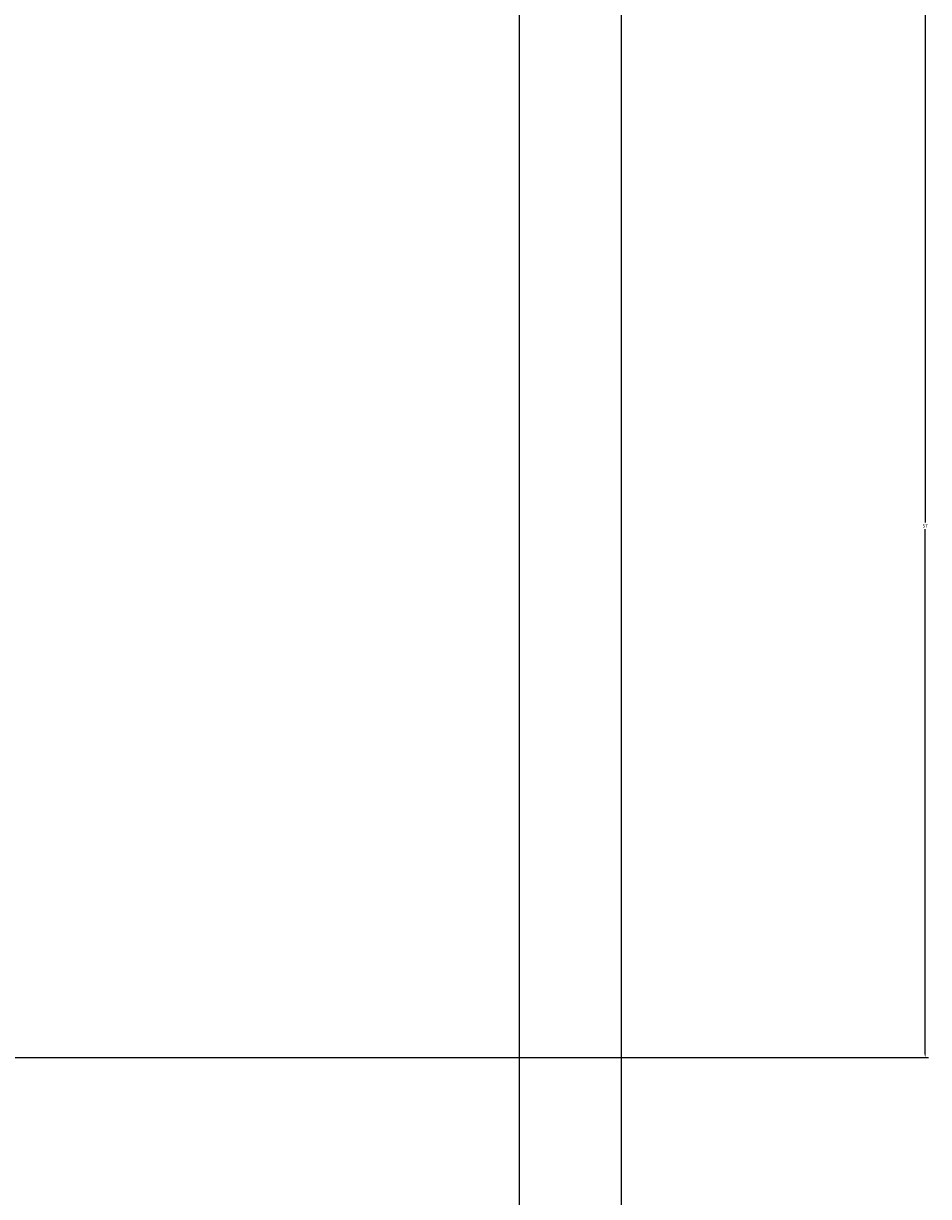
# Model space of a CAD drawing. Units: inches. Extents: x 84 to 1044, y -280 to 906.
# Tile 46 of 105: x 995 to 1044, y -129 to -66. Entities that reach past the tile are written whole.
import ezdxf

# ---------------------------------------------------------------- set-up
doc = ezdxf.new("R2010")
doc.units = ezdxf.units.IN
doc.layers.add('A-ANNO-DIMS', color=2, linetype='Continuous', lineweight=18)
doc.layers.add('A-ANNO-TTLB', color=7, linetype='Continuous', lineweight=25)
doc.styles.get("Standard").update_dxf_attribs({"font": 'arial.ttf'})
doc.dimstyles.get("Standard").update_dxf_attribs({"dimtxt": 0.18, "dimasz": 0.18, "dimexe": 0.18, "dimexo": 0.0625, "dimgap": 0.09, "dimtad": 0, "dimtih": 1, "dimtoh": 1, "dimdec": 4, "dimzin": 0, "dimdsep": 46, "dimtxsty": 'Standard', "dimcen": 0.09, "dimadec": 0, "dimazin": 0, "dimtfac": 1, "dimtdec": 4, "dimtofl": 0, "dimtmove": 0, "dimatfit": 3, "dimfxl": 1, "dimtolj": 1, "dimtzin": 0, "dimarcsym": 0})

# ---------------------------------------------------------------- blocks, each defined once
blk = doc.blocks.new('*D70')
at = {"layer": 'A-ANNO-DIMS', "color": 0, "lineweight": -2, "transparency": 16777216}
for p, q in [((983.136, -64.88), (1043.768, -64.88)), ((1043.588, -65.06), (1043.588, -93.198)), ((1043.588, -121.7), (1043.588, -93.561)), ((992.136, -121.88), (1043.768, -121.88))]:
    blk.add_line(p, q, dxfattribs=at)
at = {"layer": 'A-ANNO-DIMS', "color": 0, "transparency": 16777216}
for points in [[(1043.558, -65.06), (1043.618, -65.06), (1043.588, -64.88)], [(1043.558, -121.7), (1043.618, -121.7), (1043.588, -121.88)]]:
    blk.add_solid(points, dxfattribs=at)
at = {"layer": 'Defpoints', "color": 0, "transparency": 16777216}
for p in [(983.074, -64.88), (1043.588, -64.88), (992.074, -121.88)]:
    blk.add_point(p, dxfattribs=at)
at = {"layer": 'A-ANNO-DIMS', "color": 0, "transparency": 16777216, "insert": (1043.588, -93.38), "char_height": 0.18, "attachment_point": 5}
blk.add_mtext('\\A1;57', dxfattribs=at)

msp = doc.modelspace()

# ---------------------------------------------------------------- linework, layer by layer
at = {"layer": 'A-ANNO-TTLB'}
for points in [[(101.1, 905.916), (1027.308, 905.916), (1027.308, -279.764), (101.1, -279.764)], [(106.576, 900.439), (1021.832, 900.439), (1021.832, -274.288), (106.576, -274.288)]]:
    msp.add_lwpolyline(points, close=True, dxfattribs=at)

# ---------------------------------------------------------------- dimensions: what is measured, and where the dimension line sits
at = {"layer": 'A-ANNO-DIMS'}
dim = msp.add_linear_dim(base=(1043.588, -64.88), p1=(992.074, -121.88), p2=(983.074, -64.88), angle=90, dimstyle='Standard', override={"dimdec": 0, "dimlfac": 1, "dimrnd": 0, "dimzin": 0, "dimdsep": 46, "dimlunit": 2}, dxfattribs=at)
dim.commit()
dim.dimension.update_dxf_attribs({"geometry": '*D70', "text_midpoint": (1043.588, -93.38)})

doc.saveas('drawing.dxf')
